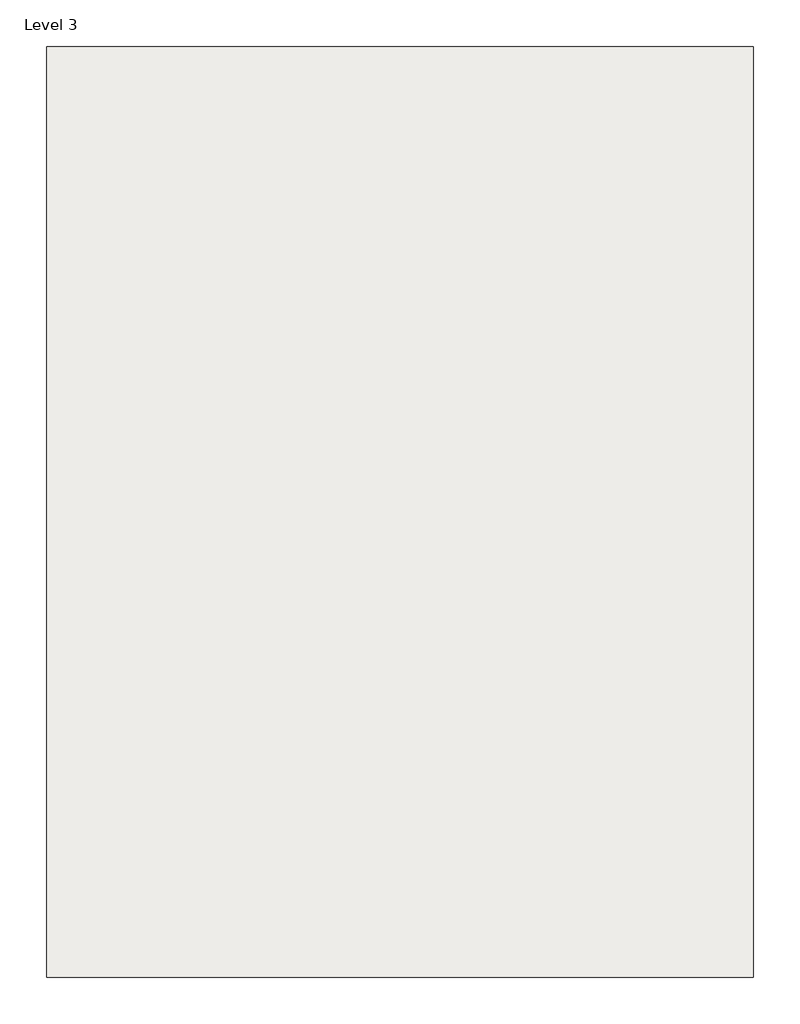
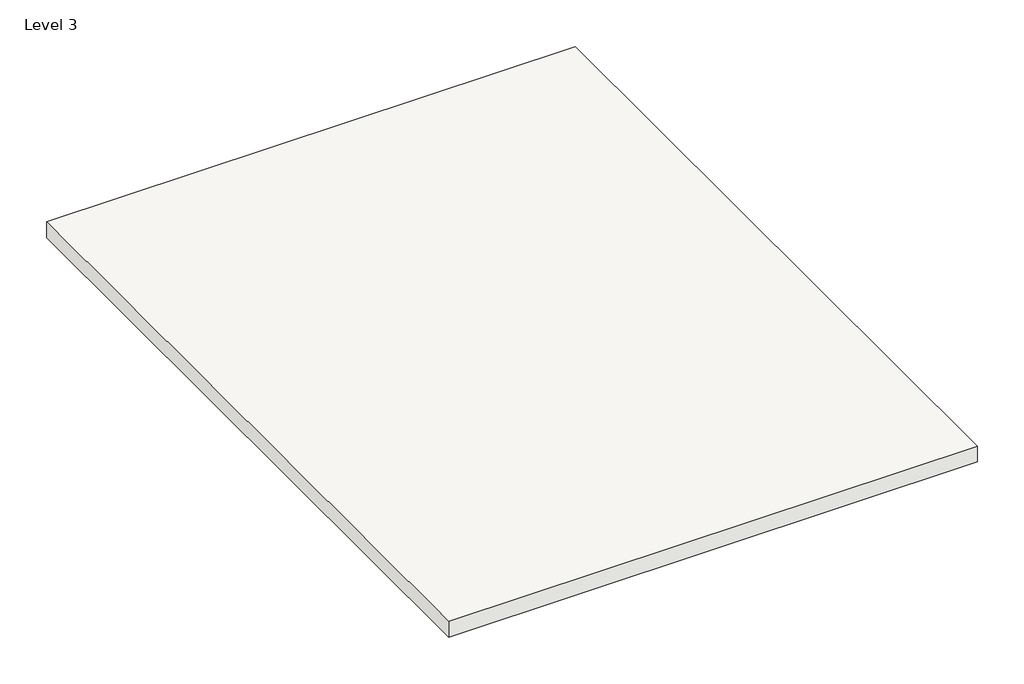
# One storey: 1 roof.
"""IFC4 building model written with IfcOpenShell, lengths in millimetres."""

from ifc_helpers import new_model, si_unit, frame, origin, place, context, project, spatial, polyline, outline, extrude, element, save

model = new_model("IFC4")

# Units and contexts
model_context = context("Model", 3, world=origin())
ifc_project = project(units=[si_unit("LENGTHUNIT", "METRE", prefix="MILLI")], contexts=[model_context])

# Site, building, storey
site = spatial("IfcSite", under=ifc_project)
building = spatial("IfcBuilding", under=site)
storey = spatial("IfcBuildingStorey", under=building, Name="Level 3", Elevation=6096.0)

# Roof
placement = place(None, origin())
element("IfcRoof", 1, ObjectType="Generic - 12\"", at=placement, inside=storey, context=model_context, shape_type="SweptSolid", body=[
    extrude(outline(polyline([(-18527.0628107, -1167.0642965), (-8925.8628107, -1167.0642965), (-8925.8628107, -13816.2642965), (-18527.0628107, -13816.2642965), (-18527.0628107, -1167.0642965)])), frame((0.0, 0.0, 6096.0), z_axis=(0.0, 0.0, 1.0), x_axis=(1.0, 0.0, 0.0)), (0.0, 0.0, 1.0), 304.8),
])

save(model, "model.ifc")

# Revit data of these elements
# Type "Generic - 12\""
#   Assembly Code = "B1020"
#   Layers, outside or top first: 1' - 0" no material (function 1)
# Element 1 (IfcRoof, "Generic - 12\"")
#   built-in parameter 1001705 = 21 (stored number, unit not read)
#   built-in parameter 1001710 = 33615
#   Phase Created = New Construction
#   Materials on its faces: "Default Roof"
# Materials
#   "Default Roof": colour RGB 88 101 114, transparency 0, Cost = 0
